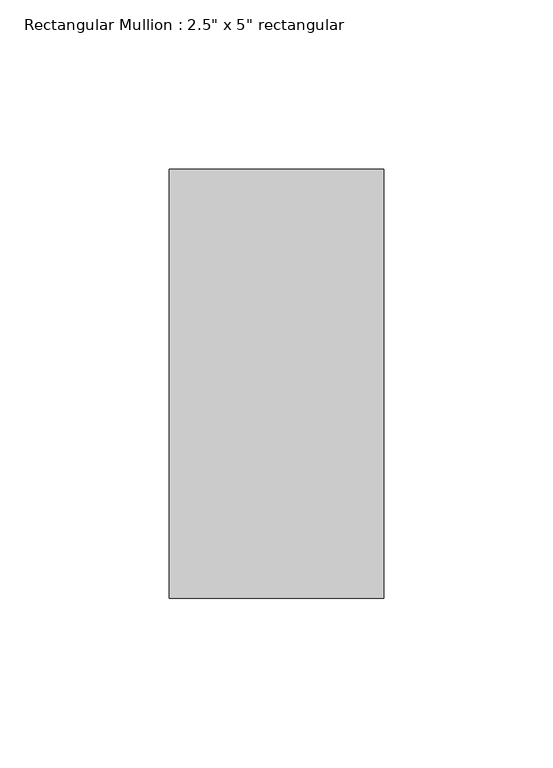
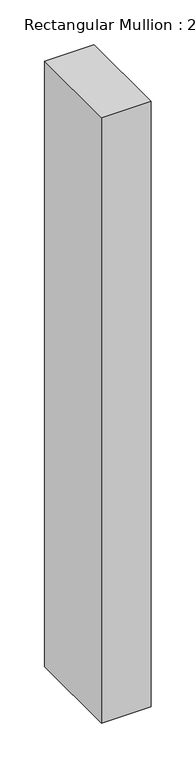
"""IFC4 building model written with IfcOpenShell, lengths in millimetres: member geometry."""

from ifc_helpers import new_model, si_unit, frame, origin, place, context, project, spatial, polyline, outline, extrude, source, transform, mapped, element, save


def member_4edd9ee4(model_context):
    return source(origin(), model_context, "Body", "SweptSolid", [
        extrude(outline(polyline([(0.0, 63.5), (0.0, -63.5), (-63.5, -63.5), (-63.5, 63.5), (0.0, 63.5)])), frame((0.0, 0.0, -823.5438093), z_axis=(0.0, 0.0, 1.0), x_axis=(1.0, 0.0, 0.0)), (0.0, 0.0, 1.0), 823.5438093),
    ])


if __name__ == "__main__":
    model = new_model("IFC4")
    model_context = context("Model", 3, world=origin())
    ifc_project = project(units=[si_unit("LENGTHUNIT", "METRE", prefix="MILLI")], contexts=[model_context])
    site = spatial("IfcSite", under=ifc_project)
    building = spatial("IfcBuilding", under=site)
    placement = place(None, origin())
    member_shape = member_4edd9ee4(model_context)
    element("IfcMember", 1, ObjectType="Rectangular Mullion : 2.5\" x 5\" rectangular", at=placement, inside=building, context=model_context, shape_type="MappedRepresentation", body=[
        mapped(member_shape, transform((0.0, 0.0, 0.0), x_axis=(1.0, 0.0, 0.0), y_axis=(0.0, 1.0, 0.0), z_axis=(0.0, 0.0, 1.0))),
    ])
    save(model, "model.ifc")

# Revit data of these elements
# Type "Rectangular Mullion : 2.5\" x 5\" rectangular"
#   built-in parameter 1007304 = 0.416667 (stored number, unit not read)
#   built-in parameter 1007301 = 0.104167 (stored number, unit not read)
#   built-in parameter 1007300 = 0.104167 (stored number, unit not read)
# Element 1 (IfcMember, "Rectangular Mullion : 2.5\" x 5\" rectangular")
#   Materials on its faces: "Aluminum"
# Materials
#   "Aluminum": class "Metal", colour RGB 247 247 247, transparency 0, Description = "Aluminum 6061", Cost = 0
